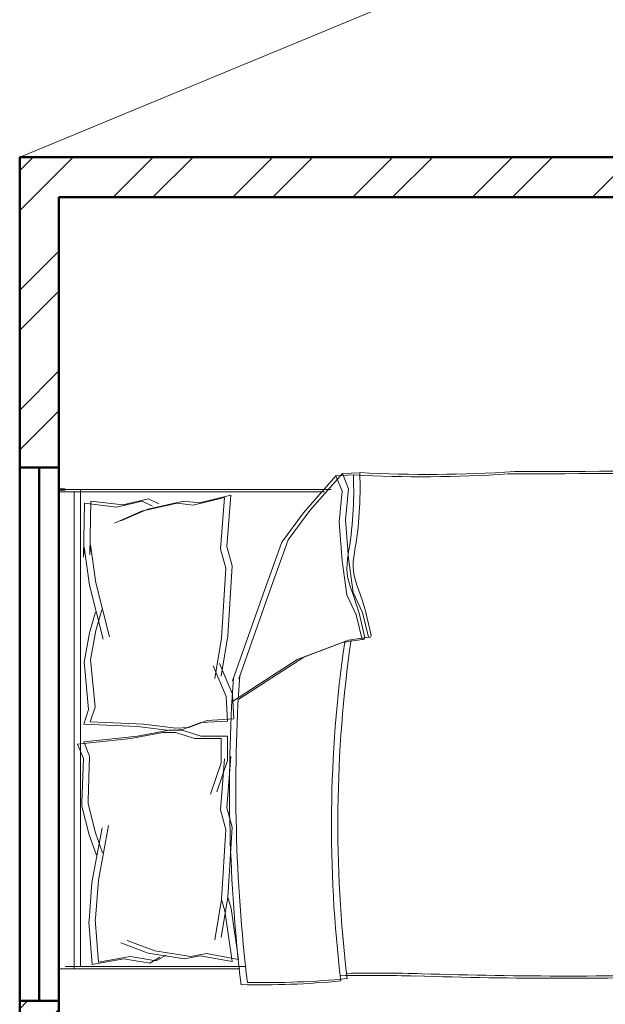
# Model space of a CAD drawing. Units: inches. Extents: x 1901 to 2863, y 888 to 2433.
# Tile 16 of 91: x 2025 to 2091, y 1621 to 1732. Entities that reach past the tile are written whole.
import ezdxf

# ---------------------------------------------------------------- set-up
doc = ezdxf.new("R2010")
doc.units = ezdxf.units.IN
for name, color, linetype, lineweight in [('A-ANNO-SYMB', 8, 'Continuous', 13), ('A-FURN', 8, 'Continuous', 18), ('A-WALL', 7, 'Continuous', 50), ('A-WALL-PATT', 8, 'Continuous', 13)]:
    doc.layers.add(name, color=color, linetype=linetype, lineweight=lineweight)

# ---------------------------------------------------------------- blocks, each defined once
blk = doc.blocks.new('BED-DOUBLE')
for p, q in [((31.18, 59.32), (27.53, 55.16)), ((31.18, 59.32), (27.53, 55.16)), ((31.9, 59.58), (28.25, 55.42)), ((31.9, 59.58), (28.25, 55.42)), ((33.14, 59.41), (31.18, 59.32, 4.35)), ((33.14, 59.41), (31.18, 59.32, 4.35)), ((31.87, 57.59), (31.18, 59.32)), ((31.87, 57.59), (31.18, 59.32)), ((33.85, 59.67), (31.9, 59.58, 4.35)), ((33.85, 59.67), (31.9, 59.58, 4.35)), ((32.59, 57.85), (31.9, 59.58)), ((32.59, 57.85), (31.9, 59.58)), ((0.03, 57.78), (0.03, 4.12)), ((0.74, 57.78), (30.62, 57.78)), ((0.74, 57.78), (30.62, 57.78)), ((32.24, 54.37), (32.59, 57.85)), ((32.24, 54.37), (32.59, 57.85)), ((7.22, 56.06), (10.11, 56.73)), ((7.22, 56.06), (10.11, 56.73)), ((10.11, 56.73), (11.28, 56.15)), ((10.11, 56.73), (11.28, 56.15)), ((18.63, 56.89), (15.11, 56.01)), ((18.63, 56.88), (15.11, 56.01)), ((19.35, 57.14), (15.83, 56.27)), ((19.35, 57.14), (15.83, 56.27)), ((18.18, 51.12), (18.63, 56.89)), ((18.18, 51.12), (18.63, 56.88)), ((18.9, 51.38), (19.35, 57.14)), ((18.9, 51.38), (19.35, 57.14)), ((31.53, 54.12), (31.87, 57.59)), ((31.53, 54.12), (31.87, 57.59)), ((2.9, 56.23), (2.79, 50.16)), ((2.9, 56.23), (2.79, 50.16)), ((2.9, 56.23), (6.5, 55.8)), ((2.9, 56.23), (6.5, 55.8)), ((3.61, 56.48), (3.51, 50.42)), ((3.61, 56.48), (3.51, 50.42)), ((3.61, 56.48), (7.22, 56.06)), ((3.61, 56.48), (7.22, 56.06)), ((6.5, 55.8), (9.39, 56.47)), ((6.5, 55.8), (9.39, 56.47)), ((10.01, 55.58), (7.01, 54.26)), ((10.01, 55.58), (7.01, 54.26)), ((13.31, 56.23), (9.3, 55.33)), ((13.31, 56.23), (9.3, 55.33)), ((9.39, 56.47), (10.56, 55.89)), ((9.39, 56.47), (10.56, 55.89)), ((14.02, 56.48), (10.01, 55.58)), ((14.02, 56.48), (10.01, 55.58)), ((15.11, 56.01), (13.31, 56.23)), ((15.11, 56.01), (13.31, 56.23)), ((15.83, 56.27), (14.02, 56.48)), ((15.83, 56.27), (14.02, 56.48)), ((28.25, 55.42), (25.81, 52.11)), ((28.25, 55.42), (25.81, 52.11)), ((9.3, 55.33), (6.29, 54)), ((9.3, 55.33), (6.29, 54)), ((27.53, 55.16), (25.1, 51.86)), ((27.53, 55.16), (25.1, 51.86)), ((32.59, 50.03), (32.24, 54.37)), ((32.59, 50.03), (32.24, 54.37)), ((31.87, 49.77), (31.53, 54.12)), ((31.87, 49.77), (31.53, 54.12)), ((25.81, 52.11), (23.55, 45.85)), ((25.81, 52.11), (23.55, 45.85)), ((2.79, 50.16), (2.88, 51.29)), ((2.79, 50.16), (2.88, 51.29)), ((2.88, 51.29), (3.47, 47.02)), ((2.88, 51.29), (3.47, 47.02)), ((3.51, 50.42), (3.6, 51.54)), ((3.51, 50.42), (3.6, 51.54)), ((3.6, 51.54), (4.19, 47.28)), ((3.6, 51.54), (4.19, 47.28)), ((18.81, 48.92), (18.18, 51.12)), ((18.81, 48.92), (18.18, 51.12)), ((19.52, 49.18), (18.9, 51.38)), ((19.52, 49.18), (18.9, 51.38)), ((25.1, 51.86), (22.84, 45.6)), ((25.1, 51.86), (22.84, 45.6)), ((33.11, 46.2), (32.59, 50.03)), ((33.11, 46.2), (32.59, 50.03)), ((18.32, 41.05), (18.81, 48.92)), ((18.32, 41.05), (18.81, 48.92)), ((19.04, 41.31), (19.52, 49.18)), ((19.04, 41.31), (19.52, 49.18)), ((32.39, 45.94), (31.87, 49.77)), ((32.39, 45.94), (31.87, 49.77)), ((3.47, 47.02), (4.99, 40.94)), ((3.47, 47.02), (4.99, 40.94)), ((4.19, 47.28), (5.71, 41.19)), ((4.19, 47.28), (5.71, 41.19)), ((22.84, 45.6), (19.54, 36.24)), ((22.84, 45.6), (19.54, 36.24)), ((23.55, 45.85), (20.26, 36.49)), ((23.55, 45.85), (20.26, 36.49)), ((33.44, 43.68), (32.39, 45.94)), ((33.44, 43.68), (32.39, 45.94)), ((34.15, 43.94), (33.11, 46.2)), ((34.15, 43.94), (33.11, 46.2)), ((89, 16.88), (89, 44.51)), ((89, 16.88), (89, 44.51)), ((89.72, 17.13), (89.72, 44.77)), ((89.72, 17.13), (89.72, 44.77)), ((4.15, 43.98), (3.48, 41.66)), ((4.15, 43.98), (3.48, 41.66)), ((4.87, 44.23), (4.2, 41.91)), ((4.87, 44.23), (4.2, 41.91)), ((34.13, 40.9), (33.44, 43.68)), ((34.13, 40.9), (33.44, 43.68)), ((34.85, 41.16), (34.15, 43.94)), ((34.85, 41.16), (34.15, 43.94)), ((3.48, 41.66), (2.87, 38.37)), ((3.48, 41.66), (2.87, 38.37)), ((4.2, 41.91), (3.59, 38.62)), ((4.2, 41.91), (3.59, 38.62)), ((17.57, 36.53), (18.32, 41.05)), ((17.57, 36.52), (18.32, 41.05)), ((18.29, 36.78), (19.04, 41.31)), ((18.29, 36.78), (19.04, 41.31)), ((32.59, 40.81), (34.85, 41.16)), ((32.59, 40.81), (34.85, 41.16)), ((26.83, 38.64), (31.87, 40.55)), ((26.83, 38.64), (31.87, 40.55)), ((27.55, 38.9), (32.59, 40.81)), ((27.55, 38.9), (32.59, 40.81)), ((31.87, 40.55), (34.13, 40.9)), ((31.87, 40.55), (34.13, 40.9)), ((20.26, 34.19), (27.55, 38.9)), ((20.26, 34.19), (27.55, 38.9)), ((2.87, 38.37), (2.9, 38.01)), ((2.87, 38.37), (2.9, 38.01)), ((2.9, 38.01), (3.37, 33.03)), ((2.9, 38.01), (3.37, 33.04)), ((3.59, 38.62), (3.62, 38.26)), ((3.59, 38.62), (3.62, 38.26)), ((3.62, 38.26), (4.09, 33.29)), ((3.62, 38.26), (4.09, 33.29)), ((18.82, 34.49), (17.38, 37.94)), ((18.82, 34.49), (17.38, 37.94)), ((19.54, 34.74), (18.1, 38.19)), ((19.54, 34.74), (18.1, 38.19)), ((19.54, 33.94), (26.83, 38.64)), ((19.54, 33.94), (26.83, 38.64)), ((18.99, 31.73), (18.82, 34.49)), ((18.99, 31.73), (18.82, 34.49)), ((19.71, 31.99), (19.54, 34.74)), ((19.71, 31.99), (19.54, 34.74)), ((4.09, 33.29), (3.54, 31.63)), ((4.09, 33.29), (3.54, 31.63)), ((3.37, 33.04), (2.82, 31.37)), ((3.37, 33.03), (2.82, 31.37)), ((2.82, 31.37), (8.86, 31.1)), ((2.82, 31.37), (8.86, 31.1)), ((3.54, 31.63), (9.58, 31.36)), ((3.54, 31.63), (9.58, 31.36)), ((8.86, 31.1), (12.46, 30.68)), ((8.86, 31.1), (12.46, 30.68)), ((9.58, 31.36), (13.18, 30.93)), ((9.58, 31.36), (13.18, 30.93)), ((13.18, 30.93), (14.64, 31.02)), ((13.18, 30.93), (14.64, 31.02)), ((13.92, 30.77), (15.99, 31.55)), ((13.92, 30.77), (15.99, 31.55)), ((14.64, 31.02), (16.71, 31.8)), ((14.64, 31.02), (16.71, 31.8)), ((15.99, 31.55), (18.99, 31.73)), ((15.99, 31.55), (18.99, 31.73)), ((16.71, 31.8), (19.71, 31.99)), ((16.71, 31.8), (19.71, 31.99)), ((2.84, 29.39), (8.85, 30.04)), ((2.84, 29.39), (8.85, 30.04)), ((8.13, 29.78), (11.7, 30.43)), ((8.13, 29.78), (11.7, 30.43)), ((8.85, 30.04), (12.42, 30.69)), ((8.85, 30.04), (12.42, 30.69)), ((11.7, 30.43), (13.16, 30.43)), ((11.7, 30.43), (13.16, 30.43)), ((12.42, 30.69), (13.88, 30.69)), ((12.42, 30.69), (13.88, 30.69)), ((12.46, 30.68), (13.92, 30.77)), ((12.46, 30.68), (13.92, 30.77)), ((13.16, 30.43), (15.28, 29.78)), ((13.16, 30.43), (15.28, 29.78)), ((13.88, 30.69), (15.99, 30.04)), ((13.88, 30.69), (15.99, 30.04)), ((15.99, 30.04), (19, 30.04)), ((15.99, 30.04), (19, 30.04)), ((19, 30.04), (19, 27.28)), ((19, 30.04), (19, 27.28)), ((2.13, 29.14), (8.13, 29.78)), ((2.13, 29.14), (8.13, 29.78)), ((2.78, 27.51), (2.13, 29.14)), ((2.78, 27.51), (2.13, 29.14)), ((3.49, 27.77), (2.84, 29.39)), ((3.49, 27.77), (2.84, 29.39)), ((15.28, 29.78), (18.29, 29.78)), ((15.28, 29.78), (18.29, 29.78)), ((18.29, 29.78), (18.29, 27.03)), ((18.29, 29.78), (18.29, 27.03)), ((3.33, 22.78), (3.49, 27.77)), ((3.33, 22.78), (3.49, 27.77)), ((18.9, 21.98), (19.35, 27.75)), ((18.9, 21.98), (19.35, 27.74)), ((2.61, 22.52), (2.78, 27.51)), ((2.61, 22.52), (2.78, 27.51)), ((18.29, 27.03), (17.06, 23.49)), ((18.29, 27.03), (17.06, 23.5)), ((19, 27.28), (17.78, 23.75)), ((19, 27.28), (17.78, 23.75)), ((18.18, 21.73), (18.63, 27.49)), ((18.18, 21.73), (18.63, 27.49)), ((2.61, 22.16), (2.61, 22.52)), ((2.61, 22.16), (2.61, 22.52)), ((3.42, 18.91), (2.61, 22.16)), ((3.42, 18.91), (2.61, 22.16)), ((3.33, 22.42), (3.33, 22.78)), ((3.33, 22.42), (3.33, 22.78)), ((4.14, 19.17), (3.33, 22.42)), ((4.14, 19.17), (3.33, 22.42)), ((18.81, 19.53), (18.18, 21.73)), ((18.81, 19.53), (18.18, 21.73)), ((19.52, 19.78), (18.9, 21.98)), ((19.52, 19.78), (18.9, 21.98)), ((4.47, 13.81), (5.6, 19.98)), ((4.47, 13.81), (5.6, 19.98)), ((4.24, 16.64), (3.42, 18.91)), ((4.24, 16.64), (3.42, 18.91)), ((3.75, 13.56), (4.89, 19.73)), ((3.75, 13.56), (4.89, 19.73)), ((4.95, 16.9), (4.14, 19.17)), ((4.95, 16.9), (4.14, 19.17)), ((18.32, 11.66), (18.81, 19.53)), ((18.32, 11.66), (18.81, 19.53)), ((19.04, 11.91), (19.52, 19.78)), ((19.04, 11.91), (19.52, 19.78)), ((3.42, 9.27), (3.75, 13.56)), ((3.42, 9.27), (3.75, 13.56)), ((4.14, 9.52), (4.47, 13.81)), ((4.14, 9.52), (4.47, 13.81)), ((17.57, 7.13), (18.32, 11.66)), ((17.57, 7.13), (18.32, 11.66)), ((18.29, 7.38), (19.04, 11.91)), ((18.29, 7.39), (19.04, 11.91)), ((18.32, 11.66), (18.68, 10.38)), ((18.32, 11.66), (18.68, 10.38)), ((19.04, 11.91), (19.4, 10.64)), ((19.04, 11.91), (19.4, 10.64)), ((18.68, 10.38), (19.5, 4.66)), ((18.68, 10.38), (19.5, 4.66)), ((19.4, 10.64), (20.21, 4.92)), ((19.4, 10.64), (20.21, 4.92)), ((3.4, 9.15), (3.42, 9.27)), ((3.4, 9.15), (3.42, 9.27)), ((3.77, 4.34), (3.4, 9.15)), ((3.77, 4.34), (3.4, 9.15)), ((4.12, 9.4), (4.14, 9.52)), ((4.12, 9.4), (4.14, 9.52)), ((4.49, 4.6), (4.12, 9.4)), ((4.49, 4.6), (4.12, 9.4)), ((10.08, 5.63), (7, 6.77)), ((10.08, 5.63), (7, 6.77)), ((10.8, 5.89), (7.71, 7.03)), ((10.8, 5.89), (7.71, 7.03)), ((14.14, 4.99), (10.08, 5.63)), ((14.14, 4.99), (10.08, 5.63)), ((14.86, 5.24), (10.8, 5.89)), ((14.86, 5.24), (10.8, 5.89)), ((16.64, 5.57), (14.86, 5.24)), ((16.64, 5.57), (14.86, 5.24)), ((20.21, 4.92), (16.64, 5.57)), ((20.21, 4.92), (16.64, 5.57)), ((3.75, 4.34), (7.32, 4.99)), ((3.75, 4.34), (7.32, 4.99)), ((4.47, 4.59), (8.04, 5.24)), ((4.47, 4.59), (8.04, 5.24)), ((7.32, 4.99), (10.24, 4.5)), ((7.32, 4.99), (10.24, 4.5)), ((8.04, 5.24), (10.96, 4.75)), ((8.04, 5.24), (10.96, 4.76)), ((10.24, 4.5), (11.38, 5.15)), ((10.24, 4.5), (11.38, 5.15)), ((10.96, 4.76), (12.1, 5.4)), ((10.96, 4.75), (12.1, 5.4)), ((15.92, 5.31), (14.14, 4.99)), ((15.92, 5.31), (14.14, 4.99)), ((19.5, 4.66), (15.92, 5.31)), ((19.5, 4.66), (15.92, 5.31))]:
    blk.add_line(p, q)
for centre, radius, start, end in [((77.12, 85.47), 25.9, 267.4714, 296.4681), ((77.12, 85.47), 25.9, 267.4714, 296.4681), ((77.84, 85.73), 25.9, 267.4714, 296.4681), ((77.84, 85.73), 25.9, 267.4714, 296.4681), ((88.58, 61.05), 1.24, 332.6588, 86.02), ((88.58, 61.05), 1.24, 332.6588, 86.02), ((89.3, 61.31), 1.24, 332.6588, 86.02), ((89.3, 61.31), 1.24, 332.6588, 86.02), ((76.89, -5061.97), 5121.82, 90.00217, 90.28689), ((76.89, -5061.97), 5121.82, 90.00217, 90.28689), ((238.36, 46.17), 149.37, 174.4998, 180.6351), ((238.36, 46.17), 149.37, 174.4998, 180.6351), ((239.08, 46.42), 149.37, 174.4998, 180.6351), ((239.08, 46.42), 149.37, 174.4998, 180.6351), ((-7.45, 57.59), 40.62, 349.8763, 2.5657), ((-7.45, 57.59), 40.62, 349.8763, 2.5657), ((40.8, 204.6), 145.39, 266.9791, 273.8365), ((40.8, 204.6), 145.39, 266.9791, 273.8365), ((-6.73, 57.85), 40.62, 349.8763, 2.5657), ((-6.73, 57.85), 40.62, 349.8763, 2.5657), ((41.52, 204.86), 145.39, 266.9791, 273.8365), ((41.52, 204.86), 145.39, 266.9791, 273.8365), ((76.17, -5062.23), 5121.82, 90.00217, 90.28689), ((76.17, -5062.23), 5121.82, 90.00217, 90.28689), ((39.4, 49.08), 6.99, 168.6608, 203.7384), ((39.4, 49.08), 6.99, 168.6608, 203.7384), ((40.11, 49.33), 6.99, 168.6608, 203.7384), ((40.11, 49.33), 6.99, 168.6608, 203.7384), ((1.69, 34.94), 33.29, 10.6617, 19.8806), ((1.69, 34.94), 33.29, 10.6617, 19.8806), ((2.41, 35.2), 33.29, 10.6617, 19.8806), ((2.41, 35.2), 33.29, 10.6617, 19.8806), ((34.2, 41.1), 0.207, 250.2464, 1.1377), ((34.2, 41.1), 0.207, 250.2464, 1.1377), ((34.92, 41.35), 0.207, 250.2464, 1.1377), ((34.92, 41.35), 0.207, 250.2464, 1.1377), ((175.53, 19.9), 144.86, 171.7845, 186.9006), ((175.53, 19.9), 144.86, 171.7845, 186.9006), ((176.25, 20.16), 144.86, 171.7845, 186.9006), ((176.25, 20.15), 144.86, 171.7845, 186.9006), ((204.43, 23.94), 185.22, 176.0865, 186.7821), ((204.43, 23.94), 185.22, 176.0865, 186.7821), ((205.14, 24.2), 185.22, 176.0865, 186.7821), ((205.14, 24.2), 185.22, 176.0865, 186.7821), ((225.52, 24.02), 136.7, 182.9958, 189.4091), ((225.52, 24.02), 136.7, 182.9958, 189.4091), ((226.23, 24.28), 136.7, 182.9958, 189.4091), ((226.23, 24.28), 136.7, 182.9958, 189.4091), ((35.74, -187.62), 190.99, 88.4762, 91.0082), ((35.74, -187.62), 190.99, 88.4762, 91.0082), ((22.59, 95.58), 93.53, 268.7218, 275.604), ((22.59, 95.58), 93.53, 268.7218, 275.604), ((23.31, 95.84), 93.53, 268.7218, 275.604), ((23.31, 95.84), 93.53, 268.7218, 275.604), ((35.03, -187.88), 190.99, 88.4762, 91.0082), ((35.03, -187.88), 190.99, 88.4762, 91.0082), ((56.85, 544.3), 541.51, 268.2277, 271.7185), ((56.85, 544.3), 541.51, 268.2277, 271.7185), ((57.57, 544.55), 541.51, 268.2277, 271.7185), ((57.57, 544.55), 541.51, 268.2277, 271.7185), ((72.46, -30.24), 33.27, 76.0648, 88.9113), ((72.46, -30.24), 33.27, 76.0648, 88.9113), ((73.18, -29.98), 33.27, 76.0648, 88.9113), ((73.18, -29.98), 33.27, 76.0648, 88.9113), ((79.65, -24.1), 26.45, 67.9751, 86.652), ((79.65, -24.1), 26.45, 67.9751, 86.652), ((78.93, -24.35), 26.45, 67.9751, 86.652), ((78.93, -24.35), 26.45, 67.9751, 86.652), ((89.53, 1.18), 1.22, 236.1736, 23.4781), ((89.53, 1.18), 1.22, 236.1736, 23.4781), ((90.25, 1.44), 1.22, 236.1736, 23.4781), ((90.25, 1.44), 1.22, 236.1736, 23.4781)]:
    blk.add_arc(centre, radius, start, end)

msp = doc.modelspace()

# ---------------------------------------------------------------- hatches: boundary and pattern name
at = {"layer": 'A-WALL-PATT'}
h = msp.add_hatch(dxfattribs=at)
h.set_pattern_fill('ANSI32', color=256)
h.paths.add_polyline_path([(2182.93, 1716.63), (2024.93, 1716.63), (2024.93, 1681.7), (2029.33, 1681.7), (2029.33, 1712.13), (2154.33, 1712.13), (2154.33, 1580.13), (2148.52, 1580.13), (2148.52, 1577.88), (2148.52, 1575.63), (2194.93, 1575.63), (2194.93, 1580.13), (2158.83, 1580.13), (2158.83, 1712.13), (2182.93, 1712.13)])
h.paths.add_polyline_path([(2301.07, 1716.63), (2242.93, 1716.63), (2242.93, 1712.13), (2283.83, 1712.13), (2283.83, 1685.54), (2288.33, 1685.54), (2288.33, 1712.13), (2301.07, 1712.13)])
h.paths.add_polyline_path([(2288.33, 1600.41), (2286.08, 1600.41), (2283.83, 1600.41), (2283.83, 1580.13), (2270.6, 1580.13), (2270.6, 1575.63), (2288.33, 1575.63)])
h.paths.add_polyline_path([(2295.93, 1953.63), (2271.45, 1953.63), (2271.45, 1949.13), (2291.43, 1949.13), (2291.43, 1941.24), (2295.93, 1941.24)])
h.paths.add_polyline_path([(2098.38, 1244.13), (2082.33, 1244.13), (2082.33, 1302.13), (2086.52, 1302.13), (2086.52, 1306.63), (2067.46, 1306.63), (2067.46, 1302.13), (2077.83, 1302.13), (2077.83, 1239.63), (2098.38, 1239.63), (2098.38, 1241.88)])
h.paths.add_polyline_path([(2217.31, 1306.63), (2158.83, 1306.63), (2158.83, 1451.63), (2162.72, 1451.63), (2162.72, 1453.88), (2162.72, 1456.13), (2154.33, 1456.13), (2154.33, 1443.13), (2151.91, 1443.13), (2151.91, 1438.63), (2154.33, 1438.63), (2154.33, 1306.63), (2109.31, 1306.63), (2109.31, 1304.38), (2109.31, 1302.13), (2154.33, 1302.13), (2154.33, 1244.13), (2122.38, 1244.13), (2122.38, 1239.63), (2154.33, 1239.63), (2154.33, 1223.63), (2163.33, 1223.63), (2181.01, 1223.63), (2181.01, 1225.88), (2181.01, 1228.13), (2163.33, 1228.13), (2163.33, 1258.22), (2158.83, 1258.22), (2158.83, 1302.13), (2217.31, 1302.13)])
h.paths.add_polyline_path([(2259.99, 1306.63), (2238.3, 1306.63), (2238.3, 1304.38), (2238.3, 1302.13), (2242.83, 1302.13), (2242.83, 1228.13), (2205.01, 1228.13), (2205.01, 1223.63), (2247.33, 1223.63), (2247.33, 1302.13), (2259.99, 1302.13), (2259.99, 1304.38)])
h.paths.add_polyline_path([(2343.43, 1361.7), (2338.93, 1361.7), (2338.93, 1306.63), (2322.38, 1306.63), (2322.38, 1302.13), (2343.43, 1302.13)])
h.paths.add_polyline_path([(2343.43, 1470.4), (2338.93, 1470.4), (2338.93, 1456.13), (2193.73, 1456.13), (2193.73, 1453.88), (2193.73, 1451.63), (2338.93, 1451.63), (2338.93, 1421.7), (2343.43, 1421.7)])
h.paths.add_polyline_path([(2343.43, 1545.51), (2338.93, 1545.51), (2338.93, 1530.4), (2343.43, 1530.4)])
h.paths.add_polyline_path([(2029.33, 1466.83), (2024.93, 1466.83), (2024.93, 1409.82), (2029.33, 1409.82)])
h.paths.add_polyline_path([(2122.84, 1440.88), (2122.84, 1443.13), (2121.83, 1443.13), (2121.83, 1498.18), (2119.58, 1498.18), (2117.33, 1498.18), (2117.33, 1443.13), (2029.33, 1443.13), (2029.33, 1438.63), (2122.84, 1438.63)])
h.paths.add_polyline_path([(2029.33, 1543.05), (2024.93, 1543.05), (2024.93, 1502.83), (2029.33, 1502.83)])
h.paths.add_polyline_path([(2029.33, 1621.7), (2024.93, 1621.7), (2024.93, 1567.05), (2027.13, 1567.05), (2029.33, 1567.05), (2029.33, 1575.63), (2109.33, 1575.63), (2109.33, 1554.71), (2113.83, 1554.71), (2113.83, 1575.63), (2115.8, 1575.63), (2115.8, 1577.88), (2115.8, 1580.13), (2029.33, 1580.13)])
h.paths.add_polyline_path([(2121.83, 1527.63), (2117.33, 1527.63), (2113.83, 1527.63), (2113.83, 1533.01), (2111.58, 1533.01), (2109.33, 1533.01), (2109.33, 1527.63), (2029.33, 1527.63), (2029.33, 1523.13), (2117.33, 1523.13), (2117.33, 1519.43), (2121.83, 1519.43)])
h.paths.add_polyline_path([(2029.33, 1349.82), (2024.93, 1349.82), (2024.93, 1302.13), (2036.28, 1302.13), (2036.28, 1306.63), (2029.33, 1306.63)])

# ---------------------------------------------------------------- linework, layer by layer
at = {"layer": 'A-ANNO-SYMB'}
msp.add_line((2256.71, 1812.63), (2024.93, 1716.63), dxfattribs=at)
at = {"layer": 'A-FURN'}
for p, q in [((2029.33, 1678.97), (2059.2, 1678.97)), ((2029.33, 1678.97), (2059.2, 1678.97)), ((2031.05, 1625.31), (2031.05, 1678.97)), ((2031.05, 1625.31), (2031.05, 1678.97)), ((2031.77, 1625.57), (2031.77, 1679.22)), ((2031.77, 1625.57), (2031.77, 1679.22)), ((2049.66, 1625.31), (2029.33, 1625.31)), ((2049.66, 1625.31), (2029.33, 1625.31)), ((2050.38, 1625.57), (2030.04, 1625.57)), ((2050.38, 1625.57), (2030.04, 1625.57))]:
    msp.add_line(p, q, dxfattribs=at)
at = {"layer": 'A-WALL'}
for p, q in [((2024.93, 1716.63), (2301.07, 1716.63)), ((2024.93, 1716.63), (2024.93, 1302.13)), ((2029.33, 1712.13), (2029.33, 1580.13)), ((2154.33, 1712.13), (2029.33, 1712.13)), ((2024.93, 1681.7), (2024.93, 1681.7)), ((2024.93, 1681.7), (2029.33, 1681.7)), ((2029.33, 1681.7), (2027.13, 1681.7)), ((2027.13, 1681.7), (2027.13, 1621.7)), ((2029.33, 1679.22), (2030.04, 1679.22)), ((2029.33, 1621.7), (2024.93, 1621.7)), ((2027.13, 1621.7), (2029.33, 1621.7))]:
    msp.add_line(p, q, dxfattribs=at)

# ---------------------------------------------------------------- block references
at = {"layer": 'A-FURN'}
msp.add_blockref('BED-DOUBLE', (2029.3, 1621.45), dxfattribs=at)

doc.saveas('drawing.dxf')
